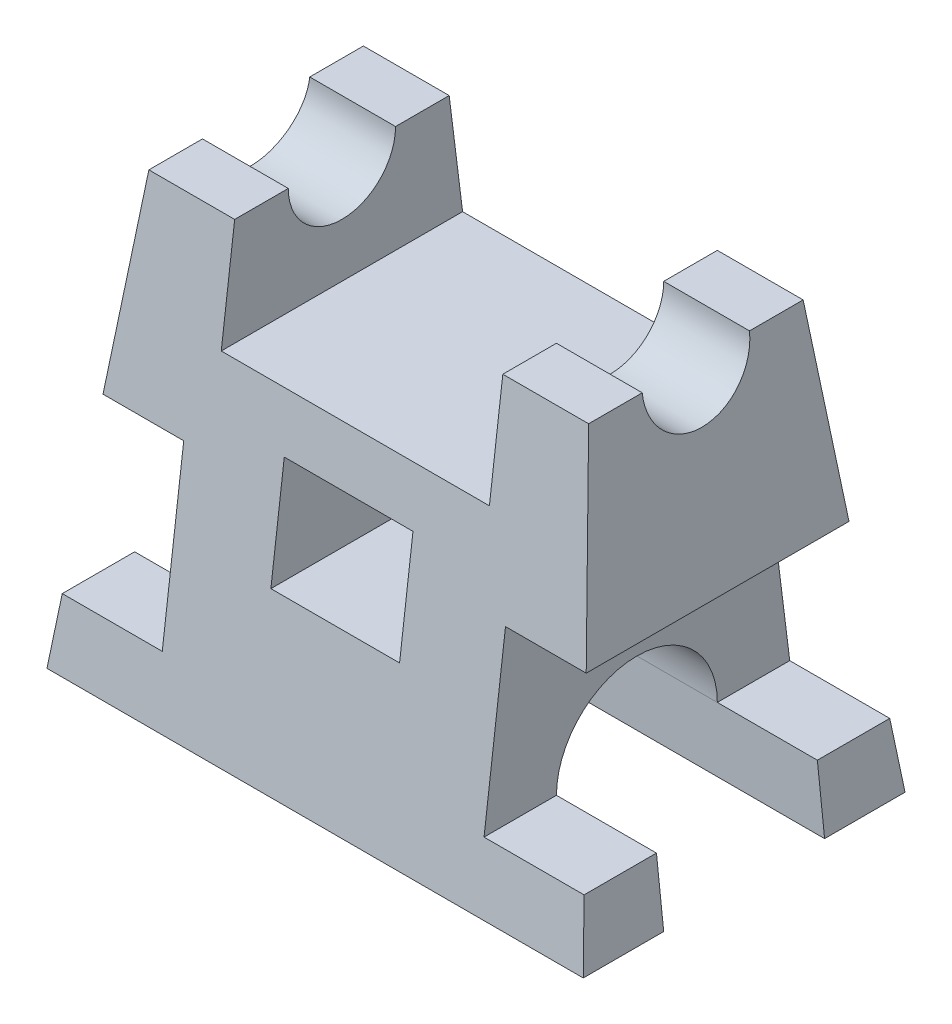
ISO-10303-21;
HEADER;
FILE_DESCRIPTION(('STEP AP214'),'2;1');
FILE_NAME('part.step','',(''),(''),'','','');
FILE_SCHEMA(('AUTOMOTIVE_DESIGN { 1 0 10303 214 1 1 1 1 }'));
ENDSEC;
DATA;
#1=APPLICATION_CONTEXT('core data for automotive mechanical design processes');
#2=APPLICATION_PROTOCOL_DEFINITION('international standard','automotive_design',2000,#1);
#3=PRODUCT_CONTEXT('',#1,'mechanical');
#4=PRODUCT('Part','Part','',(#3));
#5=PRODUCT_RELATED_PRODUCT_CATEGORY('part','',(#4));
#6=PRODUCT_DEFINITION_FORMATION('','',#4);
#7=PRODUCT_DEFINITION_CONTEXT('part definition',#1,'design');
#8=PRODUCT_DEFINITION('design','',#6,#7);
#9=PRODUCT_DEFINITION_SHAPE('','',#8);
#10=(LENGTH_UNIT() NAMED_UNIT(*) SI_UNIT(.MILLI.,.METRE.));
#11=(NAMED_UNIT(*) PLANE_ANGLE_UNIT() SI_UNIT($,.RADIAN.));
#12=(NAMED_UNIT(*) SI_UNIT($,.STERADIAN.) SOLID_ANGLE_UNIT());
#13=UNCERTAINTY_MEASURE_WITH_UNIT(LENGTH_MEASURE(1.E-05),#10,'distance_accuracy_value','');
#14=(GEOMETRIC_REPRESENTATION_CONTEXT(3) GLOBAL_UNCERTAINTY_ASSIGNED_CONTEXT((#13)) GLOBAL_UNIT_ASSIGNED_CONTEXT((#10,
#11,#12)) REPRESENTATION_CONTEXT('',''));
#15=CARTESIAN_POINT('',(0.,0.,0.));
#16=DIRECTION('',(0.,0.,1.));
#17=DIRECTION('',(1.,0.,0.));
#18=AXIS2_PLACEMENT_3D('',#15,#16,#17);
#19=CARTESIAN_POINT('',(-49.3750964357352,5.5546983490202,0.));
#20=DIRECTION('',(0.993731316158802,-0.111794773067865,0.));
#21=DIRECTION('',(0.111794773067865,0.993731316158802,0.));
#22=AXIS2_PLACEMENT_3D('',#19,#20,#21);
#23=PLANE('',#22);
#24=DIRECTION('',(0.,0.,1.));
#25=VECTOR('',#24,1.);
#26=CARTESIAN_POINT('',(-50.,0.,30.));
#27=LINE('',#26,#25);
#28=CARTESIAN_POINT('',(-50.,0.,-30.));
#29=VERTEX_POINT('',#28);
#30=CARTESIAN_POINT('',(-50.,0.,-15.));
#31=VERTEX_POINT('',#30);
#32=EDGE_CURVE('E642',#29,#31,#27,.T.);
#33=ORIENTED_EDGE('',*,*,#32,.T.);
#34=DIRECTION('',(0.111794773067865,0.993731316158802,0.));
#35=VECTOR('',#34,1.);
#36=CARTESIAN_POINT('',(-49.3750964357352,5.5546983490202,-15.));
#37=LINE('',#36,#35);
#38=CARTESIAN_POINT('',(-48.65,12.,-15.));
#39=VERTEX_POINT('',#38);
#40=EDGE_CURVE('E288',#31,#39,#37,.T.);
#41=ORIENTED_EDGE('',*,*,#40,.T.);
#42=DIRECTION('',(0.,0.,-1.));
#43=VECTOR('',#42,1.);
#44=CARTESIAN_POINT('',(-48.65,12.,0.));
#45=LINE('',#44,#43);
#46=CARTESIAN_POINT('',(-48.65,12.,-28.5));
#47=VERTEX_POINT('',#46);
#48=EDGE_CURVE('E449',#39,#47,#45,.T.);
#49=ORIENTED_EDGE('',*,*,#48,.T.);
#50=DIRECTION('',(0.110942146428332,0.986152412696287,0.123269051587036));
#51=VECTOR('',#50,1.);
#52=CARTESIAN_POINT('',(-50.,0.,-30.));
#53=LINE('',#52,#51);
#54=EDGE_CURVE('E527',#29,#47,#53,.T.);
#55=ORIENTED_EDGE('',*,*,#54,.F.);
#56=EDGE_LOOP('',(#33,#41,#49,#55));
#57=FACE_BOUND('',#56,.T.);
#58=ADVANCED_FACE('F47',(#57),#23,.F.);
#59=CARTESIAN_POINT('',(0.,0.,0.));
#60=DIRECTION('',(0.,-1.,0.));
#61=DIRECTION('',(0.,0.,-1.));
#62=AXIS2_PLACEMENT_3D('',#59,#60,#61);
#63=PLANE('',#62);
#64=DIRECTION('',(1.,0.,0.));
#65=VECTOR('',#64,1.);
#66=CARTESIAN_POINT('',(-50.0001,0.,-15.));
#67=LINE('',#66,#65);
#68=CARTESIAN_POINT('',(50.,0.,-15.));
#69=VERTEX_POINT('',#68);
#70=EDGE_CURVE('E277',#31,#69,#67,.T.);
#71=ORIENTED_EDGE('',*,*,#70,.F.);
#72=ORIENTED_EDGE('',*,*,#32,.F.);
#73=DIRECTION('',(-1.,0.,0.));
#74=VECTOR('',#73,1.);
#75=CARTESIAN_POINT('',(-50.,0.,-30.));
#76=LINE('',#75,#74);
#77=CARTESIAN_POINT('',(50.,0.,-30.));
#78=VERTEX_POINT('',#77);
#79=EDGE_CURVE('E687',#78,#29,#76,.T.);
#80=ORIENTED_EDGE('',*,*,#79,.F.);
#81=DIRECTION('',(0.,0.,-1.));
#82=VECTOR('',#81,1.);
#83=CARTESIAN_POINT('',(50.,0.,30.));
#84=LINE('',#83,#82);
#85=EDGE_CURVE('E456',#69,#78,#84,.T.);
#86=ORIENTED_EDGE('',*,*,#85,.F.);
#87=EDGE_LOOP('',(#71,#72,#80,#86));
#88=FACE_BOUND('',#87,.T.);
#89=ADVANCED_FACE('F771',(#88),#63,.T.);
#90=CARTESIAN_POINT('',(49.3750964357352,5.55469834902023,0.));
#91=DIRECTION('',(-0.993731316158802,-0.111794773067865,0.));
#92=DIRECTION('',(0.111794773067865,-0.993731316158802,0.));
#93=AXIS2_PLACEMENT_3D('',#90,#91,#92);
#94=PLANE('',#93);
#95=DIRECTION('',(0.,0.,1.));
#96=VECTOR('',#95,1.);
#97=CARTESIAN_POINT('',(48.65,12.,0.));
#98=LINE('',#97,#96);
#99=CARTESIAN_POINT('',(48.65,12.,-28.5));
#100=VERTEX_POINT('',#99);
#101=CARTESIAN_POINT('',(48.65,12.,-15.));
#102=VERTEX_POINT('',#101);
#103=EDGE_CURVE('E416',#100,#102,#98,.T.);
#104=ORIENTED_EDGE('',*,*,#103,.T.);
#105=DIRECTION('',(0.111794773067865,-0.993731316158802,0.));
#106=VECTOR('',#105,1.);
#107=CARTESIAN_POINT('',(49.3750964357352,5.55469834902022,-15.));
#108=LINE('',#107,#106);
#109=EDGE_CURVE('E290',#102,#69,#108,.T.);
#110=ORIENTED_EDGE('',*,*,#109,.T.);
#111=ORIENTED_EDGE('',*,*,#85,.T.);
#112=DIRECTION('',(-0.110942146428332,0.986152412696287,0.123269051587036));
#113=VECTOR('',#112,1.);
#114=CARTESIAN_POINT('',(50.,0.,-30.));
#115=LINE('',#114,#113);
#116=EDGE_CURVE('E595',#78,#100,#115,.T.);
#117=ORIENTED_EDGE('',*,*,#116,.T.);
#118=EDGE_LOOP('',(#104,#110,#111,#117));
#119=FACE_BOUND('',#118,.T.);
#120=ADVANCED_FACE('F602',(#119),#94,.F.);
#121=CARTESIAN_POINT('',(30.,12.,-30.0001));
#122=DIRECTION('',(0.,-1.,0.));
#123=DIRECTION('',(1.,0.,0.));
#124=AXIS2_PLACEMENT_3D('',#121,#122,#123);
#125=PLANE('',#124);
#126=DIRECTION('',(0.,0.,1.));
#127=VECTOR('',#126,1.);
#128=CARTESIAN_POINT('',(30.,12.,-30.0001));
#129=LINE('',#128,#127);
#130=CARTESIAN_POINT('',(30.,12.,-28.5));
#131=VERTEX_POINT('',#130);
#132=CARTESIAN_POINT('',(30.,12.,-15.));
#133=VERTEX_POINT('',#132);
#134=EDGE_CURVE('E407',#131,#133,#129,.T.);
#135=ORIENTED_EDGE('',*,*,#134,.T.);
#136=DIRECTION('',(1.,0.,0.));
#137=VECTOR('',#136,1.);
#138=CARTESIAN_POINT('',(-50.0001,12.,-15.));
#139=LINE('',#138,#137);
#140=EDGE_CURVE('E275',#133,#102,#139,.T.);
#141=ORIENTED_EDGE('',*,*,#140,.T.);
#142=ORIENTED_EDGE('',*,*,#103,.F.);
#143=DIRECTION('',(1.,0.,0.));
#144=VECTOR('',#143,1.);
#145=CARTESIAN_POINT('',(0.,12.,-28.5));
#146=LINE('',#145,#144);
#147=EDGE_CURVE('E543',#131,#100,#146,.T.);
#148=ORIENTED_EDGE('',*,*,#147,.F.);
#149=EDGE_LOOP('',(#135,#141,#142,#148));
#150=FACE_BOUND('',#149,.T.);
#151=ADVANCED_FACE('F815',(#150),#125,.F.);
#152=CARTESIAN_POINT('',(-30.,12.,-30.0001));
#153=DIRECTION('',(0.,-1.,0.));
#154=DIRECTION('',(1.,0.,0.));
#155=AXIS2_PLACEMENT_3D('',#152,#153,#154);
#156=PLANE('',#155);
#157=ORIENTED_EDGE('',*,*,#48,.F.);
#158=DIRECTION('',(1.,0.,0.));
#159=VECTOR('',#158,1.);
#160=CARTESIAN_POINT('',(-30.,12.,-15.));
#161=LINE('',#160,#159);
#162=CARTESIAN_POINT('',(-30.,12.,-15.));
#163=VERTEX_POINT('',#162);
#164=EDGE_CURVE('E765',#39,#163,#161,.T.);
#165=ORIENTED_EDGE('',*,*,#164,.T.);
#166=DIRECTION('',(0.,0.,1.));
#167=VECTOR('',#166,1.);
#168=CARTESIAN_POINT('',(-30.,12.,-30.0001));
#169=LINE('',#168,#167);
#170=CARTESIAN_POINT('',(-30.,12.,-28.5));
#171=VERTEX_POINT('',#170);
#172=EDGE_CURVE('E334',#171,#163,#169,.T.);
#173=ORIENTED_EDGE('',*,*,#172,.F.);
#174=DIRECTION('',(1.,0.,0.));
#175=VECTOR('',#174,1.);
#176=CARTESIAN_POINT('',(0.,12.,-28.5));
#177=LINE('',#176,#175);
#178=EDGE_CURVE('E575',#47,#171,#177,.T.);
#179=ORIENTED_EDGE('',*,*,#178,.F.);
#180=EDGE_LOOP('',(#157,#165,#173,#179));
#181=FACE_BOUND('',#180,.T.);
#182=ADVANCED_FACE('F761',(#181),#156,.F.);
#183=CARTESIAN_POINT('',(0.,80.,0.));
#184=DIRECTION('',(0.,-1.,0.));
#185=DIRECTION('',(0.,0.,-1.));
#186=AXIS2_PLACEMENT_3D('',#183,#184,#185);
#187=PLANE('',#186);
#188=DIRECTION('',(0.,0.,1.));
#189=VECTOR('',#188,1.);
#190=CARTESIAN_POINT('',(-41.,80.,20.));
#191=LINE('',#190,#189);
#192=CARTESIAN_POINT('',(-41.,80.,-20.));
#193=VERTEX_POINT('',#192);
#194=CARTESIAN_POINT('',(-41.,80.,-10.));
#195=VERTEX_POINT('',#194);
#196=EDGE_CURVE('E526',#193,#195,#191,.T.);
#197=ORIENTED_EDGE('',*,*,#196,.T.);
#198=DIRECTION('',(1.,0.,0.));
#199=VECTOR('',#198,1.);
#200=CARTESIAN_POINT('',(-50.0001,80.,-10.));
#201=LINE('',#200,#199);
#202=CARTESIAN_POINT('',(-25.,80.,-10.));
#203=VERTEX_POINT('',#202);
#204=EDGE_CURVE('E314',#195,#203,#201,.T.);
#205=ORIENTED_EDGE('',*,*,#204,.T.);
#206=DIRECTION('',(0.,0.,1.));
#207=VECTOR('',#206,1.);
#208=CARTESIAN_POINT('',(-25.,80.,-30.0001));
#209=LINE('',#208,#207);
#210=CARTESIAN_POINT('',(-25.,80.,-20.));
#211=VERTEX_POINT('',#210);
#212=EDGE_CURVE('E342',#211,#203,#209,.T.);
#213=ORIENTED_EDGE('',*,*,#212,.F.);
#214=DIRECTION('',(-1.,0.,0.));
#215=VECTOR('',#214,1.);
#216=CARTESIAN_POINT('',(-41.,80.,-20.));
#217=LINE('',#216,#215);
#218=EDGE_CURVE('E384',#211,#193,#217,.T.);
#219=ORIENTED_EDGE('',*,*,#218,.T.);
#220=EDGE_LOOP('',(#197,#205,#213,#219));
#221=FACE_BOUND('',#220,.T.);
#222=ADVANCED_FACE('F871',(#221),#187,.F.);
#223=DIRECTION('',(0.,0.,1.));
#224=VECTOR('',#223,1.);
#225=CARTESIAN_POINT('',(25.,80.,-30.0001));
#226=LINE('',#225,#224);
#227=CARTESIAN_POINT('',(25.,80.,-20.));
#228=VERTEX_POINT('',#227);
#229=CARTESIAN_POINT('',(25.,80.,-10.));
#230=VERTEX_POINT('',#229);
#231=EDGE_CURVE('E353',#228,#230,#226,.T.);
#232=ORIENTED_EDGE('',*,*,#231,.T.);
#233=CARTESIAN_POINT('',(41.,80.,-10.));
#234=VERTEX_POINT('',#233);
#235=EDGE_CURVE('E301',#230,#234,#201,.T.);
#236=ORIENTED_EDGE('',*,*,#235,.T.);
#237=DIRECTION('',(0.,0.,-1.));
#238=VECTOR('',#237,1.);
#239=CARTESIAN_POINT('',(41.,80.,20.));
#240=LINE('',#239,#238);
#241=CARTESIAN_POINT('',(41.,80.,-20.));
#242=VERTEX_POINT('',#241);
#243=EDGE_CURVE('E523',#234,#242,#240,.T.);
#244=ORIENTED_EDGE('',*,*,#243,.T.);
#245=EDGE_CURVE('E386',#242,#228,#217,.T.);
#246=ORIENTED_EDGE('',*,*,#245,.T.);
#247=EDGE_LOOP('',(#232,#236,#244,#246));
#248=FACE_BOUND('',#247,.T.);
#249=ADVANCED_FACE('F737',(#248),#187,.F.);
#250=CARTESIAN_POINT('',(-25.,80.,10.));
#251=VERTEX_POINT('',#250);
#252=CARTESIAN_POINT('',(-25.,80.,20.));
#253=VERTEX_POINT('',#252);
#254=EDGE_CURVE('E351',#251,#253,#209,.T.);
#255=ORIENTED_EDGE('',*,*,#254,.F.);
#256=DIRECTION('',(1.,0.,0.));
#257=VECTOR('',#256,1.);
#258=CARTESIAN_POINT('',(-50.0001,80.,10.));
#259=LINE('',#258,#257);
#260=CARTESIAN_POINT('',(-41.,80.,10.));
#261=VERTEX_POINT('',#260);
#262=EDGE_CURVE('E309',#261,#251,#259,.T.);
#263=ORIENTED_EDGE('',*,*,#262,.F.);
#264=CARTESIAN_POINT('',(-41.,80.,20.));
#265=VERTEX_POINT('',#264);
#266=EDGE_CURVE('E361',#261,#265,#191,.T.);
#267=ORIENTED_EDGE('',*,*,#266,.T.);
#268=DIRECTION('',(1.,0.,0.));
#269=VECTOR('',#268,1.);
#270=CARTESIAN_POINT('',(-41.,80.,20.));
#271=LINE('',#270,#269);
#272=EDGE_CURVE('E537',#265,#253,#271,.T.);
#273=ORIENTED_EDGE('',*,*,#272,.T.);
#274=EDGE_LOOP('',(#255,#263,#267,#273));
#275=FACE_BOUND('',#274,.T.);
#276=ADVANCED_FACE('F748',(#275),#187,.F.);
#277=CARTESIAN_POINT('',(-48.65,12.,28.5));
#278=VERTEX_POINT('',#277);
#279=CARTESIAN_POINT('',(-48.65,12.,15.));
#280=VERTEX_POINT('',#279);
#281=EDGE_CURVE('E448',#278,#280,#45,.T.);
#282=ORIENTED_EDGE('',*,*,#281,.T.);
#283=DIRECTION('',(-0.111794773067865,-0.993731316158802,0.));
#284=VECTOR('',#283,1.);
#285=CARTESIAN_POINT('',(-49.3750964357352,5.5546983490202,15.));
#286=LINE('',#285,#284);
#287=CARTESIAN_POINT('',(-50.,0.,15.));
#288=VERTEX_POINT('',#287);
#289=EDGE_CURVE('E292',#280,#288,#286,.T.);
#290=ORIENTED_EDGE('',*,*,#289,.T.);
#291=CARTESIAN_POINT('',(-50.,0.,30.));
#292=VERTEX_POINT('',#291);
#293=EDGE_CURVE('E662',#288,#292,#27,.T.);
#294=ORIENTED_EDGE('',*,*,#293,.T.);
#295=DIRECTION('',(0.110942146428332,0.986152412696287,-0.123269051587036));
#296=VECTOR('',#295,1.);
#297=CARTESIAN_POINT('',(-50.,0.,30.));
#298=LINE('',#297,#296);
#299=EDGE_CURVE('E468',#292,#278,#298,.T.);
#300=ORIENTED_EDGE('',*,*,#299,.T.);
#301=EDGE_LOOP('',(#282,#290,#294,#300));
#302=FACE_BOUND('',#301,.T.);
#303=ADVANCED_FACE('F777',(#302),#23,.F.);
#304=ORIENTED_EDGE('',*,*,#243,.F.);
#305=CARTESIAN_POINT('',(41.,80.,0.));
#306=DIRECTION('',(-0.993731316158802,-0.111794773067865,0.));
#307=DIRECTION('',(0.111794773067865,-0.993731316158802,0.));
#308=AXIS2_PLACEMENT_3D('',#305,#306,#307);
#309=ELLIPSE('',#308,10.0630822812894,10.);
#310=CARTESIAN_POINT('',(41.,80.,10.));
#311=VERTEX_POINT('',#310);
#312=EDGE_CURVE('E324',#234,#311,#309,.T.);
#313=ORIENTED_EDGE('',*,*,#312,.T.);
#314=CARTESIAN_POINT('',(41.,80.,20.));
#315=VERTEX_POINT('',#314);
#316=EDGE_CURVE('E525',#315,#311,#240,.T.);
#317=ORIENTED_EDGE('',*,*,#316,.F.);
#318=DIRECTION('',(-0.110942146428332,0.986152412696287,-0.123269051587036));
#319=VECTOR('',#318,1.);
#320=CARTESIAN_POINT('',(50.,0.,30.));
#321=LINE('',#320,#319);
#322=CARTESIAN_POINT('',(45.05,44.,24.5));
#323=VERTEX_POINT('',#322);
#324=EDGE_CURVE('E580',#323,#315,#321,.T.);
#325=ORIENTED_EDGE('',*,*,#324,.F.);
#326=DIRECTION('',(0.,0.,-1.));
#327=VECTOR('',#326,1.);
#328=CARTESIAN_POINT('',(45.05,44.,0.));
#329=LINE('',#328,#327);
#330=CARTESIAN_POINT('',(45.05,44.,-24.5));
#331=VERTEX_POINT('',#330);
#332=EDGE_CURVE('E424',#323,#331,#329,.T.);
#333=ORIENTED_EDGE('',*,*,#332,.T.);
#334=EDGE_CURVE('E552',#331,#242,#115,.T.);
#335=ORIENTED_EDGE('',*,*,#334,.T.);
#336=EDGE_LOOP('',(#304,#313,#317,#325,#333,#335));
#337=FACE_BOUND('',#336,.T.);
#338=ADVANCED_FACE('F603',(#337),#94,.F.);
#339=ORIENTED_EDGE('',*,*,#316,.T.);
#340=CARTESIAN_POINT('',(25.,80.,10.));
#341=VERTEX_POINT('',#340);
#342=EDGE_CURVE('E315',#341,#311,#259,.T.);
#343=ORIENTED_EDGE('',*,*,#342,.F.);
#344=CARTESIAN_POINT('',(25.,80.,20.));
#345=VERTEX_POINT('',#344);
#346=EDGE_CURVE('E394',#341,#345,#226,.T.);
#347=ORIENTED_EDGE('',*,*,#346,.T.);
#348=EDGE_CURVE('E391',#345,#315,#271,.T.);
#349=ORIENTED_EDGE('',*,*,#348,.T.);
#350=EDGE_LOOP('',(#339,#343,#347,#349));
#351=FACE_BOUND('',#350,.T.);
#352=ADVANCED_FACE('F51',(#351),#187,.F.);
#353=DIRECTION('',(1.,0.,0.));
#354=VECTOR('',#353,1.);
#355=CARTESIAN_POINT('',(-50.0001,0.,15.));
#356=LINE('',#355,#354);
#357=CARTESIAN_POINT('',(50.,0.,15.));
#358=VERTEX_POINT('',#357);
#359=EDGE_CURVE('E283',#288,#358,#356,.T.);
#360=ORIENTED_EDGE('',*,*,#359,.T.);
#361=CARTESIAN_POINT('',(50.,0.,30.));
#362=VERTEX_POINT('',#361);
#363=EDGE_CURVE('E586',#362,#358,#84,.T.);
#364=ORIENTED_EDGE('',*,*,#363,.F.);
#365=DIRECTION('',(1.,0.,0.));
#366=VECTOR('',#365,1.);
#367=CARTESIAN_POINT('',(-50.,0.,30.));
#368=LINE('',#367,#366);
#369=EDGE_CURVE('E463',#292,#362,#368,.T.);
#370=ORIENTED_EDGE('',*,*,#369,.F.);
#371=ORIENTED_EDGE('',*,*,#293,.F.);
#372=EDGE_LOOP('',(#360,#364,#370,#371));
#373=FACE_BOUND('',#372,.T.);
#374=ADVANCED_FACE('F485',(#373),#63,.T.);
#375=CARTESIAN_POINT('',(0.,3.69230769230769,29.5384615384615));
#376=DIRECTION('',(0.,-0.124034734589209,-0.992277876713668));
#377=DIRECTION('',(0.,0.992277876713668,-0.124034734589209));
#378=AXIS2_PLACEMENT_3D('',#375,#376,#377);
#379=PLANE('',#378);
#380=DIRECTION('',(1.,0.,0.));
#381=VECTOR('',#380,1.);
#382=CARTESIAN_POINT('',(0.,50.,23.75));
#383=LINE('',#382,#381);
#384=CARTESIAN_POINT('',(-12.,50.,23.75));
#385=VERTEX_POINT('',#384);
#386=CARTESIAN_POINT('',(12.,50.,23.75));
#387=VERTEX_POINT('',#386);
#388=EDGE_CURVE('E243',#385,#387,#383,.T.);
#389=ORIENTED_EDGE('',*,*,#388,.T.);
#390=DIRECTION('',(0.,-0.992277876713668,0.124034734589209));
#391=VECTOR('',#390,1.);
#392=CARTESIAN_POINT('',(12.,3.6923076923077,29.5384615384615));
#393=LINE('',#392,#391);
#394=CARTESIAN_POINT('',(12.,30.,26.25));
#395=VERTEX_POINT('',#394);
#396=EDGE_CURVE('E266',#387,#395,#393,.T.);
#397=ORIENTED_EDGE('',*,*,#396,.T.);
#398=DIRECTION('',(-1.,0.,0.));
#399=VECTOR('',#398,1.);
#400=CARTESIAN_POINT('',(0.,30.,26.25));
#401=LINE('',#400,#399);
#402=CARTESIAN_POINT('',(-12.,30.,26.25));
#403=VERTEX_POINT('',#402);
#404=EDGE_CURVE('E262',#395,#403,#401,.T.);
#405=ORIENTED_EDGE('',*,*,#404,.T.);
#406=DIRECTION('',(0.,0.992277876713668,-0.124034734589209));
#407=VECTOR('',#406,1.);
#408=CARTESIAN_POINT('',(-12.,3.69230769230769,29.5384615384615));
#409=LINE('',#408,#407);
#410=EDGE_CURVE('E246',#403,#385,#409,.T.);
#411=ORIENTED_EDGE('',*,*,#410,.T.);
#412=EDGE_LOOP('',(#389,#397,#405,#411));
#413=FACE_BOUND('',#412,.T.);
#414=DIRECTION('',(0.,-0.992277876713668,0.124034734589209));
#415=VECTOR('',#414,1.);
#416=CARTESIAN_POINT('',(-30.,3.69230769230769,29.5384615384615));
#417=LINE('',#416,#415);
#418=CARTESIAN_POINT('',(-30.,44.,24.5));
#419=VERTEX_POINT('',#418);
#420=CARTESIAN_POINT('',(-30.,12.,28.5));
#421=VERTEX_POINT('',#420);
#422=EDGE_CURVE('E453',#419,#421,#417,.T.);
#423=ORIENTED_EDGE('',*,*,#422,.T.);
#424=DIRECTION('',(-1.,0.,0.));
#425=VECTOR('',#424,1.);
#426=CARTESIAN_POINT('',(0.,12.,28.5));
#427=LINE('',#426,#425);
#428=EDGE_CURVE('E455',#421,#278,#427,.T.);
#429=ORIENTED_EDGE('',*,*,#428,.T.);
#430=ORIENTED_EDGE('',*,*,#299,.F.);
#431=ORIENTED_EDGE('',*,*,#369,.T.);
#432=CARTESIAN_POINT('',(48.65,12.,28.5));
#433=VERTEX_POINT('',#432);
#434=EDGE_CURVE('E576',#362,#433,#321,.T.);
#435=ORIENTED_EDGE('',*,*,#434,.T.);
#436=DIRECTION('',(-1.,0.,0.));
#437=VECTOR('',#436,1.);
#438=CARTESIAN_POINT('',(0.,12.,28.5));
#439=LINE('',#438,#437);
#440=CARTESIAN_POINT('',(30.,12.,28.5));
#441=VERTEX_POINT('',#440);
#442=EDGE_CURVE('E423',#433,#441,#439,.T.);
#443=ORIENTED_EDGE('',*,*,#442,.T.);
#444=DIRECTION('',(0.,0.992277876713668,-0.124034734589209));
#445=VECTOR('',#444,1.);
#446=CARTESIAN_POINT('',(30.,3.69230769230769,29.5384615384615));
#447=LINE('',#446,#445);
#448=CARTESIAN_POINT('',(30.,44.,24.5));
#449=VERTEX_POINT('',#448);
#450=EDGE_CURVE('E336',#441,#449,#447,.T.);
#451=ORIENTED_EDGE('',*,*,#450,.T.);
#452=DIRECTION('',(1.,0.,0.));
#453=VECTOR('',#452,1.);
#454=CARTESIAN_POINT('',(0.,44.,24.5));
#455=LINE('',#454,#453);
#456=EDGE_CURVE('E430',#449,#323,#455,.T.);
#457=ORIENTED_EDGE('',*,*,#456,.T.);
#458=ORIENTED_EDGE('',*,*,#324,.T.);
#459=ORIENTED_EDGE('',*,*,#348,.F.);
#460=DIRECTION('',(0.,-0.992277876713668,0.124034734589209));
#461=VECTOR('',#460,1.);
#462=CARTESIAN_POINT('',(25.,3.69230769230769,29.5384615384615));
#463=LINE('',#462,#461);
#464=CARTESIAN_POINT('',(25.,60.,22.5));
#465=VERTEX_POINT('',#464);
#466=EDGE_CURVE('E435',#345,#465,#463,.T.);
#467=ORIENTED_EDGE('',*,*,#466,.T.);
#468=DIRECTION('',(-1.,0.,0.));
#469=VECTOR('',#468,1.);
#470=CARTESIAN_POINT('',(0.,60.,22.5));
#471=LINE('',#470,#469);
#472=CARTESIAN_POINT('',(-25.,60.,22.5));
#473=VERTEX_POINT('',#472);
#474=EDGE_CURVE('E429',#465,#473,#471,.T.);
#475=ORIENTED_EDGE('',*,*,#474,.T.);
#476=DIRECTION('',(0.,0.992277876713668,-0.124034734589209));
#477=VECTOR('',#476,1.);
#478=CARTESIAN_POINT('',(-25.,3.69230769230769,29.5384615384615));
#479=LINE('',#478,#477);
#480=EDGE_CURVE('E432',#473,#253,#479,.T.);
#481=ORIENTED_EDGE('',*,*,#480,.T.);
#482=ORIENTED_EDGE('',*,*,#272,.F.);
#483=CARTESIAN_POINT('',(-45.05,44.,24.5));
#484=VERTEX_POINT('',#483);
#485=EDGE_CURVE('E510',#484,#265,#298,.T.);
#486=ORIENTED_EDGE('',*,*,#485,.F.);
#487=DIRECTION('',(1.,0.,0.));
#488=VECTOR('',#487,1.);
#489=CARTESIAN_POINT('',(0.,44.,24.5));
#490=LINE('',#489,#488);
#491=EDGE_CURVE('E442',#484,#419,#490,.T.);
#492=ORIENTED_EDGE('',*,*,#491,.T.);
#493=EDGE_LOOP('',(#423,#429,#430,#431,#435,#443,#451,#457,#458,#459,#467,#475,#481,#482,#486,#492));
#494=FACE_BOUND('',#493,.T.);
#495=ADVANCED_FACE('F265',(#413,#494),#379,.F.);
#496=ORIENTED_EDGE('',*,*,#266,.F.);
#497=CARTESIAN_POINT('',(-41.,80.,0.));
#498=DIRECTION('',(0.993731316158802,-0.111794773067865,0.));
#499=DIRECTION('',(0.111794773067865,0.993731316158802,0.));
#500=AXIS2_PLACEMENT_3D('',#497,#498,#499);
#501=ELLIPSE('',#500,10.0630822812894,10.);
#502=EDGE_CURVE('E325',#261,#195,#501,.T.);
#503=ORIENTED_EDGE('',*,*,#502,.T.);
#504=ORIENTED_EDGE('',*,*,#196,.F.);
#505=CARTESIAN_POINT('',(-45.05,44.,-24.5));
#506=VERTEX_POINT('',#505);
#507=EDGE_CURVE('E627',#506,#193,#53,.T.);
#508=ORIENTED_EDGE('',*,*,#507,.F.);
#509=DIRECTION('',(0.,0.,1.));
#510=VECTOR('',#509,1.);
#511=CARTESIAN_POINT('',(-45.05,44.,0.));
#512=LINE('',#511,#510);
#513=EDGE_CURVE('E437',#506,#484,#512,.T.);
#514=ORIENTED_EDGE('',*,*,#513,.T.);
#515=ORIENTED_EDGE('',*,*,#485,.T.);
#516=EDGE_LOOP('',(#496,#503,#504,#508,#514,#515));
#517=FACE_BOUND('',#516,.T.);
#518=ADVANCED_FACE('F481',(#517),#23,.F.);
#519=ORIENTED_EDGE('',*,*,#363,.T.);
#520=DIRECTION('',(-0.111794773067865,0.993731316158802,0.));
#521=VECTOR('',#520,1.);
#522=CARTESIAN_POINT('',(49.3750964357352,5.55469834902023,15.));
#523=LINE('',#522,#521);
#524=CARTESIAN_POINT('',(48.65,12.,15.));
#525=VERTEX_POINT('',#524);
#526=EDGE_CURVE('E788',#358,#525,#523,.T.);
#527=ORIENTED_EDGE('',*,*,#526,.T.);
#528=EDGE_CURVE('E417',#525,#433,#98,.T.);
#529=ORIENTED_EDGE('',*,*,#528,.T.);
#530=ORIENTED_EDGE('',*,*,#434,.F.);
#531=EDGE_LOOP('',(#519,#527,#529,#530));
#532=FACE_BOUND('',#531,.T.);
#533=ADVANCED_FACE('F592',(#532),#94,.F.);
#534=CARTESIAN_POINT('',(0.,3.69230769230769,-29.5384615384615));
#535=DIRECTION('',(0.,-0.124034734589208,0.992277876713668));
#536=DIRECTION('',(0.,-0.992277876713668,-0.124034734589208));
#537=AXIS2_PLACEMENT_3D('',#534,#535,#536);
#538=PLANE('',#537);
#539=DIRECTION('',(1.,0.,0.));
#540=VECTOR('',#539,1.);
#541=CARTESIAN_POINT('',(0.,30.,-26.25));
#542=LINE('',#541,#540);
#543=CARTESIAN_POINT('',(-12.,30.,-26.25));
#544=VERTEX_POINT('',#543);
#545=CARTESIAN_POINT('',(12.,30.,-26.25));
#546=VERTEX_POINT('',#545);
#547=EDGE_CURVE('E59',#544,#546,#542,.T.);
#548=ORIENTED_EDGE('',*,*,#547,.T.);
#549=DIRECTION('',(0.,0.992277876713668,0.124034734589208));
#550=VECTOR('',#549,1.);
#551=CARTESIAN_POINT('',(12.,3.69230769230769,-29.5384615384615));
#552=LINE('',#551,#550);
#553=CARTESIAN_POINT('',(12.,50.,-23.75));
#554=VERTEX_POINT('',#553);
#555=EDGE_CURVE('E12',#546,#554,#552,.T.);
#556=ORIENTED_EDGE('',*,*,#555,.T.);
#557=DIRECTION('',(-1.,0.,0.));
#558=VECTOR('',#557,1.);
#559=CARTESIAN_POINT('',(0.,50.,-23.75));
#560=LINE('',#559,#558);
#561=CARTESIAN_POINT('',(-12.,50.,-23.75));
#562=VERTEX_POINT('',#561);
#563=EDGE_CURVE('E764',#554,#562,#560,.T.);
#564=ORIENTED_EDGE('',*,*,#563,.T.);
#565=DIRECTION('',(0.,-0.992277876713668,-0.124034734589208));
#566=VECTOR('',#565,1.);
#567=CARTESIAN_POINT('',(-12.,3.69230769230769,-29.5384615384615));
#568=LINE('',#567,#566);
#569=EDGE_CURVE('E260',#562,#544,#568,.T.);
#570=ORIENTED_EDGE('',*,*,#569,.T.);
#571=EDGE_LOOP('',(#548,#556,#564,#570));
#572=FACE_BOUND('',#571,.T.);
#573=ORIENTED_EDGE('',*,*,#54,.T.);
#574=ORIENTED_EDGE('',*,*,#178,.T.);
#575=DIRECTION('',(0.,0.992277876713668,0.124034734589208));
#576=VECTOR('',#575,1.);
#577=CARTESIAN_POINT('',(-30.,3.69230769230769,-29.5384615384615));
#578=LINE('',#577,#576);
#579=CARTESIAN_POINT('',(-30.,44.,-24.5));
#580=VERTEX_POINT('',#579);
#581=EDGE_CURVE('E572',#171,#580,#578,.T.);
#582=ORIENTED_EDGE('',*,*,#581,.T.);
#583=DIRECTION('',(-1.,0.,0.));
#584=VECTOR('',#583,1.);
#585=CARTESIAN_POINT('',(0.,44.,-24.5));
#586=LINE('',#585,#584);
#587=EDGE_CURVE('E570',#580,#506,#586,.T.);
#588=ORIENTED_EDGE('',*,*,#587,.T.);
#589=ORIENTED_EDGE('',*,*,#507,.T.);
#590=ORIENTED_EDGE('',*,*,#218,.F.);
#591=DIRECTION('',(0.,-0.992277876713668,-0.124034734589208));
#592=VECTOR('',#591,1.);
#593=CARTESIAN_POINT('',(-25.,3.69230769230768,-29.5384615384615));
#594=LINE('',#593,#592);
#595=CARTESIAN_POINT('',(-25.,60.,-22.5));
#596=VERTEX_POINT('',#595);
#597=EDGE_CURVE('E565',#211,#596,#594,.T.);
#598=ORIENTED_EDGE('',*,*,#597,.T.);
#599=DIRECTION('',(1.,0.,0.));
#600=VECTOR('',#599,1.);
#601=CARTESIAN_POINT('',(0.,60.,-22.5));
#602=LINE('',#601,#600);
#603=CARTESIAN_POINT('',(25.,60.,-22.5));
#604=VERTEX_POINT('',#603);
#605=EDGE_CURVE('E556',#596,#604,#602,.T.);
#606=ORIENTED_EDGE('',*,*,#605,.T.);
#607=DIRECTION('',(0.,0.992277876713668,0.124034734589208));
#608=VECTOR('',#607,1.);
#609=CARTESIAN_POINT('',(25.,3.69230769230768,-29.5384615384615));
#610=LINE('',#609,#608);
#611=EDGE_CURVE('E558',#604,#228,#610,.T.);
#612=ORIENTED_EDGE('',*,*,#611,.T.);
#613=ORIENTED_EDGE('',*,*,#245,.F.);
#614=ORIENTED_EDGE('',*,*,#334,.F.);
#615=DIRECTION('',(-1.,0.,0.));
#616=VECTOR('',#615,1.);
#617=CARTESIAN_POINT('',(0.,44.,-24.5));
#618=LINE('',#617,#616);
#619=CARTESIAN_POINT('',(30.,44.,-24.5));
#620=VERTEX_POINT('',#619);
#621=EDGE_CURVE('E547',#331,#620,#618,.T.);
#622=ORIENTED_EDGE('',*,*,#621,.T.);
#623=DIRECTION('',(0.,-0.992277876713668,-0.124034734589208));
#624=VECTOR('',#623,1.);
#625=CARTESIAN_POINT('',(30.,3.69230769230769,-29.5384615384615));
#626=LINE('',#625,#624);
#627=EDGE_CURVE('E539',#620,#131,#626,.T.);
#628=ORIENTED_EDGE('',*,*,#627,.T.);
#629=ORIENTED_EDGE('',*,*,#147,.T.);
#630=ORIENTED_EDGE('',*,*,#116,.F.);
#631=ORIENTED_EDGE('',*,*,#79,.T.);
#632=EDGE_LOOP('',(#573,#574,#582,#588,#589,#590,#598,#606,#612,#613,#614,#622,#628,#629,#630,#631));
#633=FACE_BOUND('',#632,.T.);
#634=ADVANCED_FACE('F605',(#572,#633),#538,.F.);
#635=CARTESIAN_POINT('',(30.,44.,-30.0001));
#636=DIRECTION('',(0.,1.,0.));
#637=DIRECTION('',(0.,0.,1.));
#638=AXIS2_PLACEMENT_3D('',#635,#636,#637);
#639=PLANE('',#638);
#640=DIRECTION('',(0.,0.,1.));
#641=VECTOR('',#640,1.);
#642=CARTESIAN_POINT('',(30.,44.,-30.0001));
#643=LINE('',#642,#641);
#644=EDGE_CURVE('E329',#620,#449,#643,.T.);
#645=ORIENTED_EDGE('',*,*,#644,.F.);
#646=ORIENTED_EDGE('',*,*,#621,.F.);
#647=ORIENTED_EDGE('',*,*,#332,.F.);
#648=ORIENTED_EDGE('',*,*,#456,.F.);
#649=EDGE_LOOP('',(#645,#646,#647,#648));
#650=FACE_BOUND('',#649,.T.);
#651=ADVANCED_FACE('F804',(#650),#639,.F.);
#652=ORIENTED_EDGE('',*,*,#528,.F.);
#653=DIRECTION('',(1.,0.,0.));
#654=VECTOR('',#653,1.);
#655=CARTESIAN_POINT('',(-50.0001,12.,15.));
#656=LINE('',#655,#654);
#657=CARTESIAN_POINT('',(30.,12.,15.));
#658=VERTEX_POINT('',#657);
#659=EDGE_CURVE('E271',#658,#525,#656,.T.);
#660=ORIENTED_EDGE('',*,*,#659,.F.);
#661=EDGE_CURVE('E415',#658,#441,#129,.T.);
#662=ORIENTED_EDGE('',*,*,#661,.T.);
#663=ORIENTED_EDGE('',*,*,#442,.F.);
#664=EDGE_LOOP('',(#652,#660,#662,#663));
#665=FACE_BOUND('',#664,.T.);
#666=ADVANCED_FACE('F799',(#665),#125,.F.);
#667=CARTESIAN_POINT('',(30.,44.,-30.0001));
#668=DIRECTION('',(-1.,0.,0.));
#669=DIRECTION('',(0.,-1.,0.));
#670=AXIS2_PLACEMENT_3D('',#667,#668,#669);
#671=PLANE('',#670);
#672=ORIENTED_EDGE('',*,*,#661,.F.);
#673=CARTESIAN_POINT('',(30.,12.,0.));
#674=DIRECTION('',(-1.,0.,0.));
#675=DIRECTION('',(0.,-1.,0.));
#676=AXIS2_PLACEMENT_3D('',#673,#674,#675);
#677=CIRCLE('',#676,15.);
#678=EDGE_CURVE('E302',#658,#133,#677,.T.);
#679=ORIENTED_EDGE('',*,*,#678,.T.);
#680=ORIENTED_EDGE('',*,*,#134,.F.);
#681=ORIENTED_EDGE('',*,*,#627,.F.);
#682=ORIENTED_EDGE('',*,*,#644,.T.);
#683=ORIENTED_EDGE('',*,*,#450,.F.);
#684=EDGE_LOOP('',(#672,#679,#680,#681,#682,#683));
#685=FACE_BOUND('',#684,.T.);
#686=ADVANCED_FACE('F802',(#685),#671,.F.);
#687=CARTESIAN_POINT('',(-25.,80.,-30.0001));
#688=DIRECTION('',(-1.,0.,0.));
#689=DIRECTION('',(0.,-1.,0.));
#690=AXIS2_PLACEMENT_3D('',#687,#688,#689);
#691=PLANE('',#690);
#692=ORIENTED_EDGE('',*,*,#212,.T.);
#693=CARTESIAN_POINT('',(-25.,80.,0.));
#694=DIRECTION('',(-1.,0.,0.));
#695=DIRECTION('',(0.,-1.,0.));
#696=AXIS2_PLACEMENT_3D('',#693,#694,#695);
#697=CIRCLE('',#696,10.);
#698=EDGE_CURVE('E317',#203,#251,#697,.T.);
#699=ORIENTED_EDGE('',*,*,#698,.T.);
#700=ORIENTED_EDGE('',*,*,#254,.T.);
#701=ORIENTED_EDGE('',*,*,#480,.F.);
#702=DIRECTION('',(0.,0.,1.));
#703=VECTOR('',#702,1.);
#704=CARTESIAN_POINT('',(-25.,60.,-30.0001));
#705=LINE('',#704,#703);
#706=EDGE_CURVE('E405',#596,#473,#705,.T.);
#707=ORIENTED_EDGE('',*,*,#706,.F.);
#708=ORIENTED_EDGE('',*,*,#597,.F.);
#709=EDGE_LOOP('',(#692,#699,#700,#701,#707,#708));
#710=FACE_BOUND('',#709,.T.);
#711=ADVANCED_FACE('F743',(#710),#691,.F.);
#712=CARTESIAN_POINT('',(25.,80.,-30.0001));
#713=DIRECTION('',(1.,0.,0.));
#714=DIRECTION('',(0.,1.,0.));
#715=AXIS2_PLACEMENT_3D('',#712,#713,#714);
#716=PLANE('',#715);
#717=ORIENTED_EDGE('',*,*,#346,.F.);
#718=CARTESIAN_POINT('',(25.,80.,0.));
#719=DIRECTION('',(1.,0.,0.));
#720=DIRECTION('',(0.,1.,0.));
#721=AXIS2_PLACEMENT_3D('',#718,#719,#720);
#722=CIRCLE('',#721,10.);
#723=EDGE_CURVE('E355',#341,#230,#722,.T.);
#724=ORIENTED_EDGE('',*,*,#723,.T.);
#725=ORIENTED_EDGE('',*,*,#231,.F.);
#726=ORIENTED_EDGE('',*,*,#611,.F.);
#727=DIRECTION('',(0.,0.,1.));
#728=VECTOR('',#727,1.);
#729=CARTESIAN_POINT('',(25.,60.,-30.0001));
#730=LINE('',#729,#728);
#731=EDGE_CURVE('E393',#604,#465,#730,.T.);
#732=ORIENTED_EDGE('',*,*,#731,.T.);
#733=ORIENTED_EDGE('',*,*,#466,.F.);
#734=EDGE_LOOP('',(#717,#724,#725,#726,#732,#733));
#735=FACE_BOUND('',#734,.T.);
#736=ADVANCED_FACE('F739',(#735),#716,.F.);
#737=CARTESIAN_POINT('',(-25.,60.,-30.0001));
#738=DIRECTION('',(0.,-1.,0.));
#739=DIRECTION('',(0.,0.,-1.));
#740=AXIS2_PLACEMENT_3D('',#737,#738,#739);
#741=PLANE('',#740);
#742=ORIENTED_EDGE('',*,*,#731,.F.);
#743=ORIENTED_EDGE('',*,*,#605,.F.);
#744=ORIENTED_EDGE('',*,*,#706,.T.);
#745=ORIENTED_EDGE('',*,*,#474,.F.);
#746=EDGE_LOOP('',(#742,#743,#744,#745));
#747=FACE_BOUND('',#746,.T.);
#748=ADVANCED_FACE('F745',(#747),#741,.F.);
#749=CARTESIAN_POINT('',(-30.,44.,-30.0001));
#750=DIRECTION('',(1.,0.,0.));
#751=DIRECTION('',(0.,1.,0.));
#752=AXIS2_PLACEMENT_3D('',#749,#750,#751);
#753=PLANE('',#752);
#754=ORIENTED_EDGE('',*,*,#172,.T.);
#755=CARTESIAN_POINT('',(-30.,12.,0.));
#756=DIRECTION('',(1.,0.,0.));
#757=DIRECTION('',(0.,1.,0.));
#758=AXIS2_PLACEMENT_3D('',#755,#756,#757);
#759=CIRCLE('',#758,15.);
#760=CARTESIAN_POINT('',(-30.,12.,15.));
#761=VERTEX_POINT('',#760);
#762=EDGE_CURVE('E296',#163,#761,#759,.T.);
#763=ORIENTED_EDGE('',*,*,#762,.T.);
#764=EDGE_CURVE('E337',#761,#421,#169,.T.);
#765=ORIENTED_EDGE('',*,*,#764,.T.);
#766=ORIENTED_EDGE('',*,*,#422,.F.);
#767=DIRECTION('',(0.,0.,1.));
#768=VECTOR('',#767,1.);
#769=CARTESIAN_POINT('',(-30.,44.,-30.0001));
#770=LINE('',#769,#768);
#771=EDGE_CURVE('E339',#580,#419,#770,.T.);
#772=ORIENTED_EDGE('',*,*,#771,.F.);
#773=ORIENTED_EDGE('',*,*,#581,.F.);
#774=EDGE_LOOP('',(#754,#763,#765,#766,#772,#773));
#775=FACE_BOUND('',#774,.T.);
#776=ADVANCED_FACE('F755',(#775),#753,.F.);
#777=ORIENTED_EDGE('',*,*,#764,.F.);
#778=DIRECTION('',(-1.,0.,0.));
#779=VECTOR('',#778,1.);
#780=CARTESIAN_POINT('',(-30.,12.,15.));
#781=LINE('',#780,#779);
#782=EDGE_CURVE('E766',#761,#280,#781,.T.);
#783=ORIENTED_EDGE('',*,*,#782,.T.);
#784=ORIENTED_EDGE('',*,*,#281,.F.);
#785=ORIENTED_EDGE('',*,*,#428,.F.);
#786=EDGE_LOOP('',(#777,#783,#784,#785));
#787=FACE_BOUND('',#786,.T.);
#788=ADVANCED_FACE('F778',(#787),#156,.F.);
#789=CARTESIAN_POINT('',(-30.,44.,-30.0001));
#790=DIRECTION('',(0.,1.,0.));
#791=DIRECTION('',(0.,0.,1.));
#792=AXIS2_PLACEMENT_3D('',#789,#790,#791);
#793=PLANE('',#792);
#794=ORIENTED_EDGE('',*,*,#513,.F.);
#795=ORIENTED_EDGE('',*,*,#587,.F.);
#796=ORIENTED_EDGE('',*,*,#771,.T.);
#797=ORIENTED_EDGE('',*,*,#491,.F.);
#798=EDGE_LOOP('',(#794,#795,#796,#797));
#799=FACE_BOUND('',#798,.T.);
#800=ADVANCED_FACE('F752',(#799),#793,.F.);
#801=CARTESIAN_POINT('',(-50.0001,80.,0.));
#802=DIRECTION('',(1.,0.,0.));
#803=DIRECTION('',(0.,0.,-1.));
#804=AXIS2_PLACEMENT_3D('',#801,#802,#803);
#805=CYLINDRICAL_SURFACE('',#804,10.);
#806=ORIENTED_EDGE('',*,*,#235,.F.);
#807=ORIENTED_EDGE('',*,*,#723,.F.);
#808=ORIENTED_EDGE('',*,*,#342,.T.);
#809=ORIENTED_EDGE('',*,*,#312,.F.);
#810=EDGE_LOOP('',(#806,#807,#808,#809));
#811=FACE_BOUND('',#810,.T.);
#812=ADVANCED_FACE('F733',(#811),#805,.F.);
#813=ORIENTED_EDGE('',*,*,#262,.T.);
#814=ORIENTED_EDGE('',*,*,#698,.F.);
#815=ORIENTED_EDGE('',*,*,#204,.F.);
#816=ORIENTED_EDGE('',*,*,#502,.F.);
#817=EDGE_LOOP('',(#813,#814,#815,#816));
#818=FACE_BOUND('',#817,.T.);
#819=ADVANCED_FACE('F854',(#818),#805,.F.);
#820=CARTESIAN_POINT('',(-50.0001,12.,0.));
#821=DIRECTION('',(1.,0.,0.));
#822=DIRECTION('',(0.,0.,-1.));
#823=AXIS2_PLACEMENT_3D('',#820,#821,#822);
#824=CYLINDRICAL_SURFACE('',#823,15.);
#825=EDGE_CURVE('E781',#761,#658,#656,.T.);
#826=ORIENTED_EDGE('',*,*,#825,.F.);
#827=ORIENTED_EDGE('',*,*,#762,.F.);
#828=EDGE_CURVE('E274',#163,#133,#139,.T.);
#829=ORIENTED_EDGE('',*,*,#828,.T.);
#830=ORIENTED_EDGE('',*,*,#678,.F.);
#831=EDGE_LOOP('',(#826,#827,#829,#830));
#832=FACE_BOUND('',#831,.T.);
#833=ADVANCED_FACE('F786',(#832),#824,.F.);
#834=CARTESIAN_POINT('',(-50.0001,0.,-15.));
#835=DIRECTION('',(0.,0.,-1.));
#836=DIRECTION('',(0.,1.,0.));
#837=AXIS2_PLACEMENT_3D('',#834,#835,#836);
#838=PLANE('',#837);
#839=ORIENTED_EDGE('',*,*,#70,.T.);
#840=ORIENTED_EDGE('',*,*,#109,.F.);
#841=ORIENTED_EDGE('',*,*,#140,.F.);
#842=ORIENTED_EDGE('',*,*,#828,.F.);
#843=ORIENTED_EDGE('',*,*,#164,.F.);
#844=ORIENTED_EDGE('',*,*,#40,.F.);
#845=EDGE_LOOP('',(#839,#840,#841,#842,#843,#844));
#846=FACE_BOUND('',#845,.T.);
#847=ADVANCED_FACE('F789',(#846),#838,.F.);
#848=CARTESIAN_POINT('',(-50.0001,12.,15.));
#849=DIRECTION('',(0.,0.,1.));
#850=DIRECTION('',(1.,0.,0.));
#851=AXIS2_PLACEMENT_3D('',#848,#849,#850);
#852=PLANE('',#851);
#853=ORIENTED_EDGE('',*,*,#782,.F.);
#854=ORIENTED_EDGE('',*,*,#825,.T.);
#855=ORIENTED_EDGE('',*,*,#659,.T.);
#856=ORIENTED_EDGE('',*,*,#526,.F.);
#857=ORIENTED_EDGE('',*,*,#359,.F.);
#858=ORIENTED_EDGE('',*,*,#289,.F.);
#859=EDGE_LOOP('',(#853,#854,#855,#856,#857,#858));
#860=FACE_BOUND('',#859,.T.);
#861=ADVANCED_FACE('F784',(#860),#852,.F.);
#862=CARTESIAN_POINT('',(12.,30.,-30.0001));
#863=DIRECTION('',(1.,0.,0.));
#864=DIRECTION('',(0.,1.,0.));
#865=AXIS2_PLACEMENT_3D('',#862,#863,#864);
#866=PLANE('',#865);
#867=DIRECTION('',(0.,0.,1.));
#868=VECTOR('',#867,1.);
#869=CARTESIAN_POINT('',(12.,50.,-30.0001));
#870=LINE('',#869,#868);
#871=EDGE_CURVE('E65',#554,#387,#870,.T.);
#872=ORIENTED_EDGE('',*,*,#871,.F.);
#873=ORIENTED_EDGE('',*,*,#555,.F.);
#874=DIRECTION('',(0.,0.,1.));
#875=VECTOR('',#874,1.);
#876=CARTESIAN_POINT('',(12.,30.,-30.0001));
#877=LINE('',#876,#875);
#878=EDGE_CURVE('E248',#546,#395,#877,.T.);
#879=ORIENTED_EDGE('',*,*,#878,.T.);
#880=ORIENTED_EDGE('',*,*,#396,.F.);
#881=EDGE_LOOP('',(#872,#873,#879,#880));
#882=FACE_BOUND('',#881,.T.);
#883=ADVANCED_FACE('F916',(#882),#866,.F.);
#884=CARTESIAN_POINT('',(-12.,30.,-30.0001));
#885=DIRECTION('',(0.,-1.,0.));
#886=DIRECTION('',(0.,0.,-1.));
#887=AXIS2_PLACEMENT_3D('',#884,#885,#886);
#888=PLANE('',#887);
#889=ORIENTED_EDGE('',*,*,#878,.F.);
#890=ORIENTED_EDGE('',*,*,#547,.F.);
#891=DIRECTION('',(0.,0.,1.));
#892=VECTOR('',#891,1.);
#893=CARTESIAN_POINT('',(-12.,30.,-30.0001));
#894=LINE('',#893,#892);
#895=EDGE_CURVE('E259',#544,#403,#894,.T.);
#896=ORIENTED_EDGE('',*,*,#895,.T.);
#897=ORIENTED_EDGE('',*,*,#404,.F.);
#898=EDGE_LOOP('',(#889,#890,#896,#897));
#899=FACE_BOUND('',#898,.T.);
#900=ADVANCED_FACE('F930',(#899),#888,.F.);
#901=CARTESIAN_POINT('',(-12.,30.,-30.0001));
#902=DIRECTION('',(-1.,0.,0.));
#903=DIRECTION('',(0.,-1.,0.));
#904=AXIS2_PLACEMENT_3D('',#901,#902,#903);
#905=PLANE('',#904);
#906=ORIENTED_EDGE('',*,*,#895,.F.);
#907=ORIENTED_EDGE('',*,*,#569,.F.);
#908=DIRECTION('',(0.,0.,1.));
#909=VECTOR('',#908,1.);
#910=CARTESIAN_POINT('',(-12.,50.,-30.0001));
#911=LINE('',#910,#909);
#912=EDGE_CURVE('E68',#562,#385,#911,.T.);
#913=ORIENTED_EDGE('',*,*,#912,.T.);
#914=ORIENTED_EDGE('',*,*,#410,.F.);
#915=EDGE_LOOP('',(#906,#907,#913,#914));
#916=FACE_BOUND('',#915,.T.);
#917=ADVANCED_FACE('F255',(#916),#905,.F.);
#918=CARTESIAN_POINT('',(-12.,50.,-30.0001));
#919=DIRECTION('',(0.,1.,0.));
#920=DIRECTION('',(0.,0.,1.));
#921=AXIS2_PLACEMENT_3D('',#918,#919,#920);
#922=PLANE('',#921);
#923=ORIENTED_EDGE('',*,*,#912,.F.);
#924=ORIENTED_EDGE('',*,*,#563,.F.);
#925=ORIENTED_EDGE('',*,*,#871,.T.);
#926=ORIENTED_EDGE('',*,*,#388,.F.);
#927=EDGE_LOOP('',(#923,#924,#925,#926));
#928=FACE_BOUND('',#927,.T.);
#929=ADVANCED_FACE('F245',(#928),#922,.F.);
#930=CLOSED_SHELL('',(#58,#89,#120,#151,#182,#222,#249,#276,#303,#338,#352,#374,#495,#518,#533,
#634,#651,#666,#686,#711,#736,#748,#776,#788,#800,#812,#819,#833,#847,#861,#883,#900,#917,#929));
#931=MANIFOLD_SOLID_BREP('B2',#930);
#932=ADVANCED_BREP_SHAPE_REPRESENTATION('',(#18,#931),#14);
#933=SHAPE_DEFINITION_REPRESENTATION(#9,#932);
ENDSEC;
END-ISO-10303-21;
